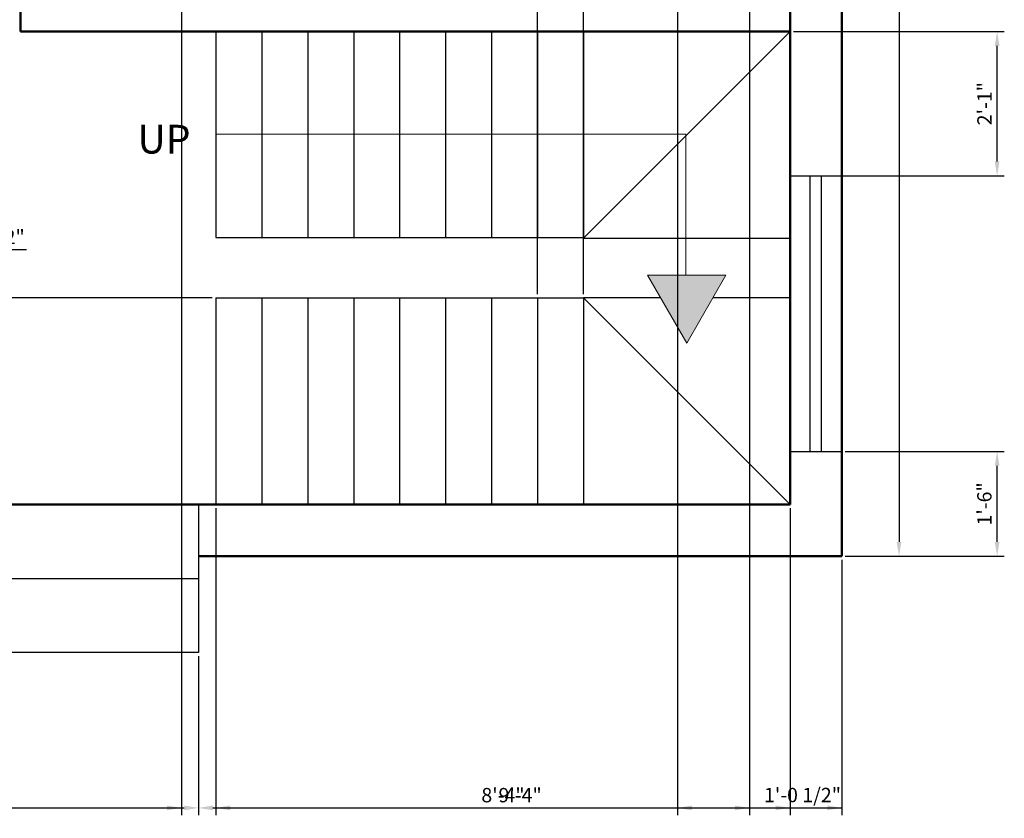
# Model space of a CAD drawing. Units: inches. Extents: x 1905 to 2315, y 3232 to 3824.
# Tile 3 of 8: x 2143 to 2314, y 3232 to 3371. Entities that reach past the tile are written whole.
import ezdxf

# ---------------------------------------------------------------- set-up
doc = ezdxf.new("R2010")
doc.units = ezdxf.units.IN
for name, color, linetype, lineweight in [('A-ANNO-DIMS', 2, 'Continuous', 18), ('A-ANNO-PATT', 7, 'Continuous', 13), ('A-ANNO-SYMB', 7, 'Continuous', 18), ('A-ANNO-TEXT', 7, 'Continuous', 18), ('A-FLOR-STRS', 7, 'Continuous', 25), ('wall', 2, 'Continuous', 50), ('WINDOW', 60, 'Continuous', 25)]:
    doc.layers.add(name, color=color, linetype=linetype, lineweight=lineweight)
doc.styles.get("Standard").update_dxf_attribs({"font": 'arial.ttf'})
doc.dimstyles.new('ISO-25', dxfattribs={"dimtxt": 2.5, "dimasz": 2.5, "dimexe": 1.25, "dimexo": 0.625, "dimtad": 1, "dimdec": 1, "dimlunit": 3, "dimtxsty": 'Standard', "dimcen": 2.5, "dimadec": 0, "dimazin": 0, "dimtfac": 1, "dimtdec": 1, "dimtmove": 0, "dimatfit": 3, "dimfxl": 1, "dimarcsym": 0})

# ---------------------------------------------------------------- blocks, each defined once
blk = doc.blocks.new('*D16')
at = {"layer": 'A-ANNO-DIMS', "color": 0, "lineweight": -2, "transparency": 16777216}
for p, q in [((2286.63, 3793.23), (2297.23, 3793.23)), ((2295.98, 3790.73), (2295.98, 3279.73)), ((2286.63, 3277.23), (2297.23, 3277.23))]:
    blk.add_line(p, q, dxfattribs=at)
at = {"layer": 'A-ANNO-DIMS', "color": 0, "transparency": 16777216}
for points in [[(2295.57, 3790.73), (2296.4, 3790.73), (2295.98, 3793.23)], [(2295.57, 3279.73), (2296.4, 3279.73), (2295.98, 3277.23)]]:
    blk.add_solid(points, dxfattribs=at)
at = {"layer": 'Defpoints', "color": 0, "transparency": 16777216}
for p in [(2286.01, 3793.23), (2286.01, 3277.23), (2295.98, 3277.23)]:
    blk.add_point(p, dxfattribs=at)
at = {"layer": 'A-ANNO-DIMS', "color": 0, "transparency": 16777216, "insert": (2294.08, 3535.23), "char_height": 2.5, "attachment_point": 5, "rotation": 90}
blk.add_mtext("43'", dxfattribs=at)
blk = doc.blocks.new('WIN-48IN')
for p, q in [((0, 9), (0, 0)), ((0, 9), (48, 9)), ((48, 9), (48, 0)), ((0, 5.5), (48, 5.5)), ((0, 3.5), (48, 3.5)), ((0, 0), (48, 0))]:
    blk.add_line(p, q)
blk = doc.blocks.new('*D41')
at = {"layer": 'A-ANNO-DIMS', "color": 0, "lineweight": -2, "transparency": 16777216}
for p, q in [((2095.01, 3663.61), (2095.01, 3232.16)), ((2171.01, 3663.61), (2171.01, 3232.16)), ((2097.51, 3233.41), (2168.51, 3233.41))]:
    blk.add_line(p, q, dxfattribs=at)
at = {"layer": 'A-ANNO-DIMS', "color": 0, "transparency": 16777216}
for points in [[(2097.51, 3233.83), (2097.51, 3233), (2095.01, 3233.41)], [(2168.51, 3233.83), (2168.51, 3233), (2171.01, 3233.41)]]:
    blk.add_solid(points, dxfattribs=at)
at = {"layer": 'Defpoints', "color": 0, "transparency": 16777216}
for p in [(2095.01, 3664.23), (2171.01, 3664.23), (2171.01, 3233.41)]:
    blk.add_point(p, dxfattribs=at)
at = {"layer": 'A-ANNO-DIMS', "color": 0, "transparency": 16777216, "insert": (2133.01, 3235.31), "char_height": 2.5, "attachment_point": 5}
blk.add_mtext('6\'-4"', dxfattribs=at)
blk = doc.blocks.new('*D49')
at = {"layer": 'A-ANNO-DIMS', "color": 0, "lineweight": -2, "transparency": 16777216}
for p, q in [((2286.63, 3295.48), (2314.32, 3295.48)), ((2313.07, 3279.73), (2313.07, 3292.98)), ((2286.63, 3277.23), (2314.32, 3277.23))]:
    blk.add_line(p, q, dxfattribs=at)
at = {"layer": 'A-ANNO-DIMS', "color": 0, "transparency": 16777216}
for points in [[(2312.65, 3292.98), (2313.48, 3292.98), (2313.07, 3295.48)], [(2312.65, 3279.73), (2313.48, 3279.73), (2313.07, 3277.23)]]:
    blk.add_solid(points, dxfattribs=at)
at = {"layer": 'Defpoints', "color": 0, "transparency": 16777216}
for p in [(2286.01, 3295.48), (2313.07, 3295.48), (2286.01, 3277.23)]:
    blk.add_point(p, dxfattribs=at)
at = {"layer": 'A-ANNO-DIMS', "color": 0, "transparency": 16777216, "insert": (2311.17, 3286.35), "char_height": 2.5, "attachment_point": 5, "rotation": 90}
blk.add_mtext('1\'-6"', dxfattribs=at)
blk = doc.blocks.new('*D50')
at = {"layer": 'A-ANNO-DIMS', "color": 0, "lineweight": -2, "transparency": 16777216}
for p, q in [((2277.63, 3368.6), (2314.32, 3368.6)), ((2313.07, 3345.98), (2313.07, 3366.1)), ((2277.63, 3343.48), (2314.32, 3343.48))]:
    blk.add_line(p, q, dxfattribs=at)
at = {"layer": 'A-ANNO-DIMS', "color": 0, "transparency": 16777216}
for points in [[(2312.65, 3366.1), (2313.48, 3366.1), (2313.07, 3368.6)], [(2312.65, 3345.98), (2313.48, 3345.98), (2313.07, 3343.48)]]:
    blk.add_solid(points, dxfattribs=at)
at = {"layer": 'Defpoints', "color": 0, "transparency": 16777216}
for p in [(2277.01, 3368.6), (2313.07, 3368.6), (2277.01, 3343.48)]:
    blk.add_point(p, dxfattribs=at)
at = {"layer": 'A-ANNO-DIMS', "color": 0, "transparency": 16777216, "insert": (2311.19, 3356.04), "char_height": 2.5, "attachment_point": 5, "rotation": 90}
blk.add_mtext('2\'-1"', dxfattribs=at)
blk = doc.blocks.new('*D57')
at = {"layer": 'A-ANNO-DIMS', "color": 0, "lineweight": -2, "transparency": 16777216}
for p, q in [((2095.91, 3259.85), (2095.91, 3232.16)), ((2173.99, 3259.85), (2173.99, 3232.16)), ((2098.41, 3233.41), (2171.49, 3233.41))]:
    blk.add_line(p, q, dxfattribs=at)
at = {"layer": 'A-ANNO-DIMS', "color": 0, "transparency": 16777216}
for points in [[(2098.41, 3233.83), (2098.41, 3233), (2095.91, 3233.41)], [(2171.49, 3233.83), (2171.49, 3233), (2173.99, 3233.41)]]:
    blk.add_solid(points, dxfattribs=at)
at = {"layer": 'Defpoints', "color": 0, "transparency": 16777216}
for p in [(2095.91, 3260.47), (2173.99, 3260.47), (2173.99, 3233.41)]:
    blk.add_point(p, dxfattribs=at)
at = {"layer": 'A-ANNO-DIMS', "color": 0, "transparency": 16777216, "insert": (2134.95, 3235.31), "char_height": 2.5, "attachment_point": 5}
blk.add_mtext('6\'-6"', dxfattribs=at)
blk = doc.blocks.new('*D58')
at = {"layer": 'A-ANNO-DIMS', "color": 0, "lineweight": -2, "transparency": 16777216}
for p, q in [((2286.01, 3276.61), (2286.01, 3232.16)), ((2173.99, 3259.85), (2173.99, 3232.16)), ((2176.49, 3233.41), (2283.51, 3233.41))]:
    blk.add_line(p, q, dxfattribs=at)
at = {"layer": 'A-ANNO-DIMS', "color": 0, "transparency": 16777216}
for points in [[(2176.49, 3233.83), (2176.49, 3233), (2173.99, 3233.41)], [(2283.51, 3233.83), (2283.51, 3233), (2286.01, 3233.41)]]:
    blk.add_solid(points, dxfattribs=at)
at = {"layer": 'Defpoints', "color": 0, "transparency": 16777216}
for p in [(2286.01, 3277.23), (2173.99, 3260.47), (2286.01, 3233.41)]:
    blk.add_point(p, dxfattribs=at)
at = {"layer": 'A-ANNO-DIMS', "color": 0, "transparency": 16777216, "insert": (2230, 3235.31), "char_height": 2.5, "attachment_point": 5}
blk.add_mtext('9\'-4"', dxfattribs=at)
blk = doc.blocks.new('*D60')
at = {"layer": 'A-ANNO-DIMS', "color": 0, "lineweight": -2, "transparency": 16777216}
for p, q in [((2177.01, 3285.61), (2177.01, 3232.16)), ((2277.01, 3285.61), (2277.01, 3232.16)), ((2179.51, 3233.41), (2274.51, 3233.41))]:
    blk.add_line(p, q, dxfattribs=at)
at = {"layer": 'A-ANNO-DIMS', "color": 0, "transparency": 16777216}
for points in [[(2179.51, 3233.83), (2179.51, 3233), (2177.01, 3233.41)], [(2274.51, 3233.83), (2274.51, 3233), (2277.01, 3233.41)]]:
    blk.add_solid(points, dxfattribs=at)
at = {"layer": 'Defpoints', "color": 0, "transparency": 16777216}
for p in [(2177.01, 3286.23), (2277.01, 3286.23), (2277.01, 3233.41)]:
    blk.add_point(p, dxfattribs=at)
at = {"layer": 'A-ANNO-DIMS', "color": 0, "transparency": 16777216, "insert": (2227.01, 3235.31), "char_height": 2.5, "attachment_point": 5}
blk.add_mtext('8\'-4"', dxfattribs=at)
blk = doc.blocks.new('*D61')
at = {"layer": 'A-ANNO-DIMS', "color": 0, "lineweight": -2, "transparency": 16777216}
for p, q in [((2176.38, 3322.23), (1909.7, 3322.23)), ((1910.95, 3288.73), (1910.95, 3319.73)), ((2176.38, 3286.23), (1909.7, 3286.23))]:
    blk.add_line(p, q, dxfattribs=at)
at = {"layer": 'A-ANNO-DIMS', "color": 0, "transparency": 16777216}
for points in [[(1910.53, 3319.73), (1911.36, 3319.73), (1910.95, 3322.23)], [(1910.53, 3288.73), (1911.36, 3288.73), (1910.95, 3286.23)]]:
    blk.add_solid(points, dxfattribs=at)
at = {"layer": 'Defpoints', "color": 0, "transparency": 16777216}
for p in [(1910.95, 3322.23), (2177.01, 3322.23), (2177.01, 3286.23)]:
    blk.add_point(p, dxfattribs=at)
at = {"layer": 'A-ANNO-DIMS', "color": 0, "transparency": 16777216, "insert": (1909.05, 3304.23), "char_height": 2.5, "attachment_point": 5, "rotation": 90}
blk.add_mtext('3\'-0"', dxfattribs=at)
blk = doc.blocks.new('*D62')
at = {"layer": 'A-ANNO-DIMS', "color": 0, "lineweight": -2, "transparency": 16777216}
for p, q in [((2233.01, 3322.86), (2233.01, 3821.54)), ((2241.01, 3322.86), (2241.01, 3821.54)), ((2235.51, 3820.29), (2238.51, 3820.29))]:
    blk.add_line(p, q, dxfattribs=at)
at = {"layer": 'A-ANNO-DIMS', "color": 0, "transparency": 16777216}
for points in [[(2235.51, 3820.71), (2235.51, 3819.88), (2233.01, 3820.29)], [(2238.51, 3820.71), (2238.51, 3819.88), (2241.01, 3820.29)]]:
    blk.add_solid(points, dxfattribs=at)
at = {"layer": 'Defpoints', "color": 0, "transparency": 16777216}
for p in [(2241.01, 3820.29), (2233.01, 3322.23), (2241.01, 3322.23)]:
    blk.add_point(p, dxfattribs=at)
at = {"layer": 'A-ANNO-DIMS', "color": 0, "transparency": 16777216, "insert": (2237.01, 3822.19), "char_height": 2.5, "attachment_point": 5}
blk.add_mtext('0\'-8"', dxfattribs=at)
blk = doc.blocks.new('*D68')
at = {"layer": 'A-ANNO-DIMS', "color": 0, "lineweight": -2, "transparency": 16777216}
for p, q in [((2257.4, 3401.51), (2257.4, 3232.16)), ((2269.93, 3401.51), (2269.93, 3232.16)), ((2259.9, 3233.41), (2267.43, 3233.41)), ((2269.93, 3233.41), (2285.92, 3233.41))]:
    blk.add_line(p, q, dxfattribs=at)
at = {"layer": 'A-ANNO-DIMS', "color": 0, "transparency": 16777216}
for points in [[(2259.9, 3233.83), (2259.9, 3233), (2257.4, 3233.41)], [(2267.43, 3233.83), (2267.43, 3233), (2269.93, 3233.41)]]:
    blk.add_solid(points, dxfattribs=at)
at = {"layer": 'Defpoints', "color": 0, "transparency": 16777216}
for p in [(2257.4, 3402.13), (2269.93, 3402.13), (2269.93, 3233.41)]:
    blk.add_point(p, dxfattribs=at)
at = {"layer": 'A-ANNO-DIMS', "color": 0, "transparency": 16777216, "insert": (2279.17, 3235.33), "char_height": 2.5, "attachment_point": 5}
blk.add_mtext('1\'-0 1/2"', dxfattribs=at)
blk = doc.blocks.new('*D79')
at = {"layer": 'A-ANNO-DIMS', "color": 0, "lineweight": -2, "transparency": 16777216}
for p, q in [((2001.48, 3330.59), (2084.93, 3330.59)), ((2144.02, 3330.59), (2087.43, 3330.59))]:
    blk.add_line(p, q, dxfattribs=at)
at = {"layer": 'A-ANNO-DIMS', "color": 0, "transparency": 16777216}
blk.add_solid([(2087.43, 3331.01), (2087.43, 3330.17), (2084.93, 3330.59)], dxfattribs=at)
at = {"layer": 'Defpoints', "color": 0, "transparency": 16777216}
for p in [(2001.48, 3330.59), (2084.93, 3330.59)]:
    blk.add_point(p, dxfattribs=at)
at = {"layer": 'A-ANNO-DIMS', "color": 0, "transparency": 16777216, "insert": (2134.99, 3332.51), "char_height": 2.5, "attachment_point": 5, "rotation": 0.0001}
blk.add_mtext('R6\'-11 1/2"', dxfattribs=at)

msp = doc.modelspace()

# ---------------------------------------------------------------- hatches: boundary and pattern name
at = {"layer": 'A-ANNO-PATT'}
h = msp.add_hatch(color=256, dxfattribs=at)
h.dxf.hatch_style = 1
h.paths.add_polyline_path([(2265.85, 3326.18), (2252.17, 3326.18), (2259.01, 3314.33)])

# ---------------------------------------------------------------- linework, layer by layer
at = {"layer": 'A-ANNO-SYMB'}
for p, q in [((2177.01, 3350.73), (2258.88, 3350.73)), ((2258.88, 3350.73), (2258.88, 3326.18))]:
    msp.add_line(p, q, dxfattribs=at)
msp.add_lwpolyline([(2259.01, 3314.33), (2265.85, 3326.18), (2252.17, 3326.18)], close=True, dxfattribs=at)
at = {"layer": 'A-FLOR-STRS'}
for p, q in [((2177.01, 3368.73), (2177.01, 3332.73)), ((2177.01, 3368.73), (2241.01, 3368.73)), ((2185.01, 3368.73), (2185.01, 3332.73)), ((2193.01, 3368.73), (2193.01, 3332.73)), ((2201.01, 3368.73), (2201.01, 3332.73)), ((2209.01, 3368.73), (2209.01, 3332.73)), ((2217.01, 3368.73), (2217.01, 3332.73)), ((2225.01, 3368.73), (2225.01, 3332.73)), ((2233.01, 3368.73), (2233.01, 3332.73)), ((2277.01, 3368.6), (2241.01, 3368.6)), ((2241.01, 3368.6), (2241.01, 3332.6)), ((2241.01, 3332.6), (2277.01, 3368.6)), ((2277.01, 3332.6), (2277.01, 3368.6)), ((2177.01, 3332.73), (2241.01, 3332.73)), ((2241.01, 3332.6), (2277.01, 3332.6)), ((2177.01, 3322.23), (2177.01, 3286.23)), ((2177.01, 3322.23), (2241.01, 3322.23)), ((2185.01, 3322.23), (2185.01, 3286.23)), ((2193.01, 3322.23), (2193.01, 3286.23)), ((2201.01, 3322.23), (2201.01, 3286.23)), ((2209.01, 3322.23), (2209.01, 3286.23)), ((2217.01, 3322.23), (2217.01, 3286.23)), ((2225.01, 3322.23), (2225.01, 3286.23)), ((2233.01, 3322.23), (2233.01, 3286.23)), ((2241.01, 3322.23), (2241.01, 3286.23)), ((2241.01, 3322.23), (2277.01, 3286.23)), ((2254.45, 3322.23), (2241.01, 3322.23)), ((2277.01, 3322.23), (2263.57, 3322.23)), ((2277.01, 3286.23), (2277.01, 3322.23)), ((2177.01, 3286.23), (2241.01, 3286.23)), ((2241.01, 3286.23), (2277.01, 3286.23)), ((2095.91, 3273.38), (2173.99, 3273.38))]:
    msp.add_line(p, q, dxfattribs=at)
msp.add_lwpolyline([(2095.91, 3286.29), (2173.99, 3286.29), (2173.99, 3260.47), (2095.91, 3260.47)], close=True, dxfattribs=at)
at = {"layer": 'wall'}
for p, q in [((2286.01, 3277.23), (2286.01, 3793.23)), ((2277.01, 3286.23), (2277.01, 3784.23)), ((2143.01, 3372.6), (2143.01, 3368.6)), ((2277.01, 3368.6), (2143.01, 3368.6)), ((1947.01, 3286.23), (2277.01, 3286.23)), ((2173.99, 3277.23), (2286.01, 3277.23))]:
    msp.add_line(p, q, dxfattribs=at)

# ---------------------------------------------------------------- block references
at = {"layer": 'WINDOW', "rotation": 89.99999999999793}
msp.add_blockref('WIN-48IN', (2286.01, 3295.48), dxfattribs=at)

# ---------------------------------------------------------------- texts
at = {"layer": 'A-ANNO-TEXT', "insert": (2163.36, 3352.36), "char_height": 5, "attachment_point": 1}
msp.add_mtext_dynamic_manual_height_columns('UP', width=56.1502, gutter_width=12.5, heights=[0], dxfattribs=at)

# ---------------------------------------------------------------- dimensions: what is measured, and where the dimension line sits
at = {"layer": 'A-ANNO-DIMS'}
for base, p1, p2, picture, middle in [((2241.01, 3820.29), (2233.01, 3322.23), (2241.01, 3322.23), '*D62', (2237.01, 3822.19)), ((2171.01, 3233.41), (2095.01, 3664.23), (2171.01, 3664.23), '*D41', (2133.01, 3235.31)), ((2269.93, 3233.41), (2257.4, 3402.13), (2269.93, 3402.13), '*D68', (2279.17, 3235.33)), ((2277.01, 3233.41), (2177.01, 3286.23), (2277.01, 3286.23), '*D60', (2227.01, 3235.31)), ((2286.01, 3233.41), (2173.99, 3260.47), (2286.01, 3277.23), '*D58', (2230, 3235.31)), ((2173.99, 3233.41), (2095.91, 3260.47), (2173.99, 3260.47), '*D57', (2134.95, 3235.31))]:
    dim = msp.add_linear_dim(base=base, p1=p1, p2=p2, dimstyle='ISO-25', override={"dimdec": 1, "dimlfac": 1, "dimrnd": 0, "dimzin": 1, "dimdsep": 46, "dimlunit": 4, "dimfrac": 2}, dxfattribs=at)
    dim.commit()
    dim.dimension.update_dxf_attribs({"geometry": picture, "text_midpoint": middle})
for base, p1, p2, override, picture, middle in [((2295.98, 3277.23), (2286.01, 3793.23), (2286.01, 3277.23), {"dimclrd": 0, "dimclre": 0, "dimclrt": 0}, '*D16', (2294.08, 3535.23)), ((2313.07, 3368.6), (2277.01, 3343.48), (2277.01, 3368.6), {"dimdec": 1, "dimlfac": 1, "dimrnd": 0, "dimzin": 1, "dimdsep": 46, "dimlunit": 4, "dimfrac": 2}, '*D50', (2311.19, 3356.04)), ((1910.95, 3322.23), (2177.01, 3286.23), (2177.01, 3322.23), {"dimdec": 1, "dimlfac": 1, "dimrnd": 0, "dimzin": 1, "dimdsep": 46, "dimlunit": 4, "dimfrac": 2}, '*D61', (1909.05, 3304.23)), ((2313.0676, 3295.4768), (2286.0076, 3277.2318), (2286.0076, 3295.4768), {"dimdec": 1, "dimlfac": 1, "dimrnd": 0, "dimzin": 1, "dimdsep": 46, "dimlunit": 4, "dimfrac": 2}, '*D49', (2311.1662, 3286.3543))]:
    dim = msp.add_linear_dim(base=base, p1=p1, p2=p2, angle=90, dimstyle='ISO-25', override=override, dxfattribs=at)
    dim.commit()
    dim.dimension.update_dxf_attribs({"geometry": picture, "text_midpoint": middle})
dim = msp.add_radius_dim(center=(2001.4831, 3330.5909), mpoint=(2084.9264, 3330.591), dimstyle='ISO-25', override={"dimdec": 1, "dimlfac": 1, "dimrnd": 0, "dimzin": 1, "dimdsep": 46, "dimlunit": 4, "dimfrac": 2}, dxfattribs=at)
dim.commit()
dim.dimension.update_dxf_attribs({"geometry": '*D79', "text_midpoint": (2134.9924, 3330.5911), "dimtype": 164})

doc.saveas('drawing.dxf')
